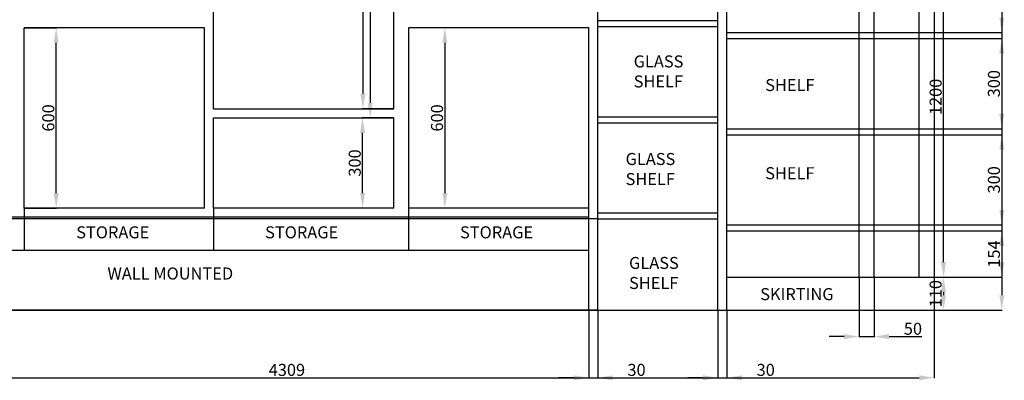
# Model space of a CAD drawing. Units: millimetres. Extents: x -2182 to 7969, y 257 to 4097.
# Tile 4 of 5: x 4692 to 7969, y 257 to 1457. Entities that reach past the tile are written whole.
import ezdxf

# ---------------------------------------------------------------- set-up
doc = ezdxf.new("R2010")
doc.units = ezdxf.units.MM
for name, color, linetype, lineweight in [('A-ANNO-DIMS', 2, 'Continuous', 18), ('A-ANNO-TEXT', 3, 'Continuous', 18), ('A-ELEV', 7, 'Continuous', 25)]:
    doc.layers.add(name, color=color, linetype=linetype, lineweight=lineweight)
doc.styles.get("Standard").update_dxf_attribs({"font": 'arial.ttf'})
doc.dimstyles.new('ISO-25', dxfattribs={"dimtxt": 40, "dimasz": 50, "dimexe": 1.25, "dimexo": 0.625, "dimtad": 1, "dimtxsty": 'Standard', "dimcen": 2.5, "dimadec": 0, "dimazin": 0, "dimtfac": 1, "dimtmove": 0, "dimatfit": 3, "dimfxl": 1, "dimarcsym": 0})

# ---------------------------------------------------------------- blocks, each defined once
blk = doc.blocks.new('*D52')
at = {"layer": 'A-ANNO-DIMS', "color": 0, "lineweight": -2, "transparency": 16777216}
for p, q in [((7686.6, 600), (7768.1, 600)), ((7766.8, 550), (7766.8, 540)), ((7686.6, 490), (7768.1, 490))]:
    blk.add_line(p, q, dxfattribs=at)
at = {"layer": 'A-ANNO-DIMS', "color": 0, "transparency": 16777216}
for points in [[(7758.5, 550), (7775.2, 550), (7766.8, 600)], [(7758.5, 540), (7775.2, 540), (7766.8, 490)]]:
    blk.add_solid(points, dxfattribs=at)
at = {"layer": 'Defpoints', "color": 0, "transparency": 16777216}
for p in [(7685.9, 600), (7685.9, 490), (7766.8, 490)]:
    blk.add_point(p, dxfattribs=at)
at = {"layer": 'A-ANNO-DIMS', "color": 0, "transparency": 16777216, "insert": (7745.8, 545), "char_height": 40, "attachment_point": 5, "rotation": 90}
blk.add_mtext('110', dxfattribs=at)
blk = doc.blocks.new('*D53')
at = {"layer": 'A-ANNO-DIMS', "color": 0, "lineweight": -2, "transparency": 16777216}
for p, q in [((7686.6, 1800), (7768.3, 1800)), ((7767.1, 650), (7767.1, 1750)), ((7536.6, 600), (7768.3, 600))]:
    blk.add_line(p, q, dxfattribs=at)
at = {"layer": 'A-ANNO-DIMS', "color": 0, "transparency": 16777216}
for points in [[(7758.7, 1750), (7775.4, 1750), (7767.1, 1800)], [(7758.7, 650), (7775.4, 650), (7767.1, 600)]]:
    blk.add_solid(points, dxfattribs=at)
at = {"layer": 'Defpoints', "color": 0, "transparency": 16777216}
for p in [(7685.9, 1800), (7767.1, 1800), (7535.9, 600)]:
    blk.add_point(p, dxfattribs=at)
at = {"layer": 'A-ANNO-DIMS', "color": 0, "transparency": 16777216, "insert": (7746, 1200), "char_height": 40, "attachment_point": 5, "rotation": 90}
blk.add_mtext('1200', dxfattribs=at)
blk = doc.blocks.new('*D54')
at = {"layer": 'A-ANNO-DIMS', "color": 0, "lineweight": -2, "transparency": 16777216}
for p, q in [((7485.9, 599.4), (7485.9, 400.8)), ((7535.9, 599.4), (7535.9, 400.8)), ((7435.9, 402.1), (7385.9, 402.1)), ((7485.9, 402.1), (7535.9, 402.1)), ((7585.9, 402.1), (7694.4, 402.1))]:
    blk.add_line(p, q, dxfattribs=at)
at = {"layer": 'A-ANNO-DIMS', "color": 0, "transparency": 16777216}
for points in [[(7435.9, 410.4), (7435.9, 393.7), (7485.9, 402.1)], [(7585.9, 410.4), (7585.9, 393.7), (7535.9, 402.1)]]:
    blk.add_solid(points, dxfattribs=at)
at = {"layer": 'Defpoints', "color": 0, "transparency": 16777216}
for p in [(7485.9, 600), (7535.9, 600), (7485.9, 402.1)]:
    blk.add_point(p, dxfattribs=at)
at = {"layer": 'A-ANNO-DIMS', "color": 0, "transparency": 16777216, "insert": (7665.2, 423.1), "char_height": 40, "attachment_point": 5}
blk.add_mtext('50', dxfattribs=at)
blk = doc.blocks.new('*D32')
at = {"layer": 'A-ANNO-DIMS', "color": 0, "lineweight": -2, "transparency": 16777216}
for p, q in [((6285.3, 1430), (6106, 1430)), ((6107.2, 1380), (6107.2, 880)), ((6285.3, 830), (6106, 830))]:
    blk.add_line(p, q, dxfattribs=at)
at = {"layer": 'A-ANNO-DIMS', "color": 0, "transparency": 16777216}
for points in [[(6098.9, 1380), (6115.6, 1380), (6107.2, 1430)], [(6098.9, 880), (6115.6, 880), (6107.2, 830)]]:
    blk.add_solid(points, dxfattribs=at)
at = {"layer": 'Defpoints', "color": 0, "transparency": 16777216}
for p in [(6285.9, 1430), (6107.2, 830), (6285.9, 830)]:
    blk.add_point(p, dxfattribs=at)
at = {"layer": 'A-ANNO-DIMS', "color": 0, "transparency": 16777216, "insert": (6086.2, 1130), "char_height": 40, "attachment_point": 5, "rotation": 90}
blk.add_mtext('600', dxfattribs=at)
blk = doc.blocks.new('*D40')
at = {"layer": 'A-ANNO-DIMS', "color": 0, "lineweight": -2, "transparency": 16777216}
for p, q in [((5936.3, 2864), (5857.3, 2864)), ((5858.6, 2814), (5858.6, 1180)), ((5936.3, 1130), (5857.3, 1130))]:
    blk.add_line(p, q, dxfattribs=at)
at = {"layer": 'A-ANNO-DIMS', "color": 0, "transparency": 16777216}
for points in [[(5850.2, 2814), (5866.9, 2814), (5858.6, 2864)], [(5850.2, 1180), (5866.9, 1180), (5858.6, 1130)]]:
    blk.add_solid(points, dxfattribs=at)
at = {"layer": 'Defpoints', "color": 0, "transparency": 16777216}
for p in [(5936.9, 2864), (5858.6, 1130), (5936.9, 1130)]:
    blk.add_point(p, dxfattribs=at)
at = {"layer": 'A-ANNO-DIMS', "color": 0, "transparency": 16777216, "insert": (5837.5, 1997), "char_height": 40, "attachment_point": 5, "rotation": 90}
blk.add_mtext('1734', dxfattribs=at)
blk = doc.blocks.new('*D33')
at = {"layer": 'A-ANNO-DIMS', "color": 0, "lineweight": -2, "transparency": 16777216}
for p, q in [((5936.3, 1997), (5833.1, 1997)), ((5834.4, 1947), (5834.4, 1210)), ((5936.3, 1160), (5833.1, 1160))]:
    blk.add_line(p, q, dxfattribs=at)
at = {"layer": 'A-ANNO-DIMS', "color": 0, "transparency": 16777216}
for points in [[(5826, 1947), (5842.7, 1947), (5834.4, 1997)], [(5826, 1210), (5842.7, 1210), (5834.4, 1160)]]:
    blk.add_solid(points, dxfattribs=at)
at = {"layer": 'Defpoints', "color": 0, "transparency": 16777216}
for p in [(5936.9, 1997), (5834.4, 1160), (5936.9, 1160)]:
    blk.add_point(p, dxfattribs=at)
at = {"layer": 'A-ANNO-DIMS', "color": 0, "transparency": 16777216, "insert": (5813.3, 1578.5), "char_height": 40, "attachment_point": 5, "rotation": 90}
blk.add_mtext('837', dxfattribs=at)
blk = doc.blocks.new('*D44')
at = {"layer": 'A-ANNO-DIMS', "color": 0, "lineweight": -2, "transparency": 16777216}
for p, q in [((5936.3, 1130), (5832.1, 1130)), ((5833.3, 880), (5833.3, 1080)), ((5936.3, 830), (5832.1, 830))]:
    blk.add_line(p, q, dxfattribs=at)
at = {"layer": 'A-ANNO-DIMS', "color": 0, "transparency": 16777216}
for points in [[(5825, 1080), (5841.7, 1080), (5833.3, 1130)], [(5825, 880), (5841.7, 880), (5833.3, 830)]]:
    blk.add_solid(points, dxfattribs=at)
at = {"layer": 'Defpoints', "color": 0, "transparency": 16777216}
for p in [(5833.3, 1130), (5936.9, 1130), (5936.9, 830)]:
    blk.add_point(p, dxfattribs=at)
at = {"layer": 'A-ANNO-DIMS', "color": 0, "transparency": 16777216, "insert": (5812.3, 980), "char_height": 40, "attachment_point": 5, "rotation": 90}
blk.add_mtext('300', dxfattribs=at)
blk = doc.blocks.new('*D47')
at = {"layer": 'A-ANNO-DIMS', "color": 0, "lineweight": -2, "transparency": 16777216}
for p, q in [((4707.6, 1430), (4814.7, 1430)), ((4813.4, 880), (4813.4, 1380)), ((4707.6, 830), (4814.7, 830))]:
    blk.add_line(p, q, dxfattribs=at)
at = {"layer": 'A-ANNO-DIMS', "color": 0, "transparency": 16777216}
for points in [[(4805.1, 1380), (4821.7, 1380), (4813.4, 1430)], [(4805.1, 880), (4821.7, 880), (4813.4, 830)]]:
    blk.add_solid(points, dxfattribs=at)
at = {"layer": 'Defpoints', "color": 0, "transparency": 16777216}
for p in [(4706.9, 1430), (4813.4, 1430), (4706.9, 830)]:
    blk.add_point(p, dxfattribs=at)
at = {"layer": 'A-ANNO-DIMS', "color": 0, "transparency": 16777216, "insert": (4792.4, 1130), "char_height": 40, "attachment_point": 5, "rotation": 90}
blk.add_mtext('600', dxfattribs=at)
blk = doc.blocks.new('*D77')
at = {"layer": 'A-ANNO-DIMS', "color": 0, "lineweight": -2, "transparency": 16777216}
for p, q in [((7735.9, 3063.4), (7735.9, 263.7)), ((3426.9, 489.4), (3426.9, 263.7)), ((3476.9, 265), (7685.9, 265))]:
    blk.add_line(p, q, dxfattribs=at)
at = {"layer": 'A-ANNO-DIMS', "color": 0, "transparency": 16777216}
for points in [[(3476.9, 273.3), (3476.9, 256.7), (3426.9, 265)], [(7685.9, 273.3), (7685.9, 256.7), (7735.9, 265)]]:
    blk.add_solid(points, dxfattribs=at)
at = {"layer": 'Defpoints', "color": 0, "transparency": 16777216}
for p in [(7735.9, 3064), (3426.9, 490), (7735.9, 265)]:
    blk.add_point(p, dxfattribs=at)
at = {"layer": 'A-ANNO-DIMS', "color": 0, "transparency": 16777216, "insert": (5581.4, 286.1), "char_height": 40, "attachment_point": 5}
blk.add_mtext('4309', dxfattribs=at)
blk = doc.blocks.new('*D79')
at = {"layer": 'A-ANNO-DIMS', "color": 0, "lineweight": -2, "transparency": 16777216}
for p, q in [((7736.6, 3164), (7962.2, 3164)), ((7960.9, 3114), (7960.9, 540)), ((3427.6, 490), (7962.2, 490))]:
    blk.add_line(p, q, dxfattribs=at)
at = {"layer": 'A-ANNO-DIMS', "color": 0, "transparency": 16777216}
for points in [[(7952.6, 3114), (7969.3, 3114), (7960.9, 3164)], [(7952.6, 540), (7969.3, 540), (7960.9, 490)]]:
    blk.add_solid(points, dxfattribs=at)
at = {"layer": 'Defpoints', "color": 0, "transparency": 16777216}
for p in [(7735.9, 3164), (3426.9, 490), (7960.9, 490)]:
    blk.add_point(p, dxfattribs=at)
at = {"layer": 'A-ANNO-DIMS', "color": 0, "transparency": 16777216, "insert": (7939.9, 1827), "char_height": 40, "attachment_point": 5, "rotation": 90}
blk.add_mtext('2674', dxfattribs=at)
blk = doc.blocks.new('*D90')
at = {"layer": 'A-ANNO-DIMS', "color": 0, "lineweight": -2, "transparency": 16777216}
for p, q in [((6585.9, 489.4), (6585.9, 263.7)), ((6615.9, 489.4), (6615.9, 263.7)), ((6535.9, 265), (6485.9, 265)), ((6585.9, 265), (6615.9, 265)), ((6665.9, 265), (6774.3, 265))]:
    blk.add_line(p, q, dxfattribs=at)
at = {"layer": 'A-ANNO-DIMS', "color": 0, "transparency": 16777216}
for points in [[(6535.9, 273.3), (6535.9, 256.7), (6585.9, 265)], [(6665.9, 273.3), (6665.9, 256.7), (6615.9, 265)]]:
    blk.add_solid(points, dxfattribs=at)
at = {"layer": 'Defpoints', "color": 0, "transparency": 16777216}
for p in [(6585.9, 490), (6615.9, 490), (6615.9, 265)]:
    blk.add_point(p, dxfattribs=at)
at = {"layer": 'A-ANNO-DIMS', "color": 0, "transparency": 16777216, "insert": (6745.1, 286.1), "char_height": 40, "attachment_point": 5}
blk.add_mtext('30', dxfattribs=at)
blk = doc.blocks.new('*D91')
at = {"layer": 'A-ANNO-DIMS', "color": 0, "lineweight": -2, "transparency": 16777216}
for p, q in [((7015.9, 489.4), (7015.9, 263.7)), ((7045.9, 489.4), (7045.9, 263.7)), ((6965.9, 265), (6915.9, 265)), ((7015.9, 265), (7045.9, 265)), ((7095.9, 265), (7204.3, 265))]:
    blk.add_line(p, q, dxfattribs=at)
at = {"layer": 'A-ANNO-DIMS', "color": 0, "transparency": 16777216}
for points in [[(6965.9, 273.3), (6965.9, 256.7), (7015.9, 265)], [(7095.9, 273.3), (7095.9, 256.7), (7045.9, 265)]]:
    blk.add_solid(points, dxfattribs=at)
at = {"layer": 'Defpoints', "color": 0, "transparency": 16777216}
for p in [(7015.9, 490), (7045.9, 490), (7045.9, 265)]:
    blk.add_point(p, dxfattribs=at)
at = {"layer": 'A-ANNO-DIMS', "color": 0, "transparency": 16777216, "insert": (7175.1, 286.1), "char_height": 40, "attachment_point": 5}
blk.add_mtext('30', dxfattribs=at)
blk = doc.blocks.new('*D95')
at = {"layer": 'A-ANNO-DIMS', "color": 0, "lineweight": -2, "transparency": 16777216}
for p, q in [((6615.3, 794), (3200.7, 794)), ((3201.9, 744), (3201.9, 540)), ((6615.3, 490), (3200.7, 490))]:
    blk.add_line(p, q, dxfattribs=at)
at = {"layer": 'A-ANNO-DIMS', "color": 0, "transparency": 16777216}
for points in [[(3193.6, 744), (3210.3, 744), (3201.9, 794)], [(3193.6, 540), (3210.3, 540), (3201.9, 490)]]:
    blk.add_solid(points, dxfattribs=at)
at = {"layer": 'Defpoints', "color": 0, "transparency": 16777216}
for p in [(6615.9, 794), (3201.9, 490), (6615.9, 490)]:
    blk.add_point(p, dxfattribs=at)
at = {"layer": 'A-ANNO-DIMS', "color": 0, "transparency": 16777216, "insert": (3180.9, 642), "char_height": 40, "attachment_point": 5, "rotation": 90}
blk.add_mtext('304', dxfattribs=at)
blk = doc.blocks.new('*D99')
at = {"layer": 'A-ANNO-DIMS', "color": 0, "lineweight": -2, "transparency": 16777216}
for p, q in [((7486.6, 1714), (7962.2, 1714)), ((7960.9, 1664), (7960.9, 1464)), ((7486.6, 1414), (7962.2, 1414))]:
    blk.add_line(p, q, dxfattribs=at)
at = {"layer": 'A-ANNO-DIMS', "color": 0, "transparency": 16777216}
for points in [[(7952.6, 1664), (7969.3, 1664), (7960.9, 1714)], [(7952.6, 1464), (7969.3, 1464), (7960.9, 1414)]]:
    blk.add_solid(points, dxfattribs=at)
at = {"layer": 'Defpoints', "color": 0, "transparency": 16777216}
for p in [(7485.9, 1714), (7485.9, 1414), (7960.9, 1414)]:
    blk.add_point(p, dxfattribs=at)
at = {"layer": 'A-ANNO-DIMS', "color": 0, "transparency": 16777216, "insert": (7939.9, 1564), "char_height": 40, "attachment_point": 5, "rotation": 90}
blk.add_mtext('300', dxfattribs=at)
blk = doc.blocks.new('*D100')
at = {"layer": 'A-ANNO-DIMS', "color": 0, "lineweight": -2, "transparency": 16777216}
for p, q in [((7486.6, 1394), (7962.2, 1394)), ((7960.9, 1344), (7960.9, 1144)), ((7486.6, 1094), (7962.2, 1094))]:
    blk.add_line(p, q, dxfattribs=at)
at = {"layer": 'A-ANNO-DIMS', "color": 0, "transparency": 16777216}
for points in [[(7952.6, 1344), (7969.3, 1344), (7960.9, 1394)], [(7952.6, 1144), (7969.3, 1144), (7960.9, 1094)]]:
    blk.add_solid(points, dxfattribs=at)
at = {"layer": 'Defpoints', "color": 0, "transparency": 16777216}
for p in [(7485.9, 1394), (7485.9, 1094), (7960.9, 1094)]:
    blk.add_point(p, dxfattribs=at)
at = {"layer": 'A-ANNO-DIMS', "color": 0, "transparency": 16777216, "insert": (7939.9, 1244), "char_height": 40, "attachment_point": 5, "rotation": 90}
blk.add_mtext('300', dxfattribs=at)
blk = doc.blocks.new('*D101')
at = {"layer": 'A-ANNO-DIMS', "color": 0, "lineweight": -2, "transparency": 16777216}
for p, q in [((7486.6, 1074), (7962.2, 1074)), ((7960.9, 1024), (7960.9, 824)), ((7486.6, 774), (7962.2, 774))]:
    blk.add_line(p, q, dxfattribs=at)
at = {"layer": 'A-ANNO-DIMS', "color": 0, "transparency": 16777216}
for points in [[(7952.6, 1024), (7969.3, 1024), (7960.9, 1074)], [(7952.6, 824), (7969.3, 824), (7960.9, 774)]]:
    blk.add_solid(points, dxfattribs=at)
at = {"layer": 'Defpoints', "color": 0, "transparency": 16777216}
for p in [(7485.9, 1074), (7485.9, 774), (7960.9, 774)]:
    blk.add_point(p, dxfattribs=at)
at = {"layer": 'A-ANNO-DIMS', "color": 0, "transparency": 16777216, "insert": (7939.9, 924), "char_height": 40, "attachment_point": 5, "rotation": 90}
blk.add_mtext('300', dxfattribs=at)
blk = doc.blocks.new('*D102')
at = {"layer": 'A-ANNO-DIMS', "color": 0, "lineweight": -2, "transparency": 16777216}
for p, q in [((7486.6, 754), (7962.2, 754)), ((7960.9, 704), (7960.9, 650)), ((7486.6, 600), (7962.2, 600))]:
    blk.add_line(p, q, dxfattribs=at)
at = {"layer": 'A-ANNO-DIMS', "color": 0, "transparency": 16777216}
for points in [[(7952.6, 704), (7969.3, 704), (7960.9, 754)], [(7952.6, 650), (7969.3, 650), (7960.9, 600)]]:
    blk.add_solid(points, dxfattribs=at)
at = {"layer": 'Defpoints', "color": 0, "transparency": 16777216}
for p in [(7485.9, 754), (7485.9, 600), (7960.9, 600)]:
    blk.add_point(p, dxfattribs=at)
at = {"layer": 'A-ANNO-DIMS', "color": 0, "transparency": 16777216, "insert": (7939.9, 677), "char_height": 40, "attachment_point": 5, "rotation": 90}
blk.add_mtext('154', dxfattribs=at)

msp = doc.modelspace()

# ---------------------------------------------------------------- linework, layer by layer
at = {"layer": 'A-ELEV'}
for p, q in [((5936.9478, 1159.9911), (5936.9478, 3163.9911)), ((7535.9478, 599.9911), (7535.9478, 3063.9911)), ((7685.9478, 599.9911), (7685.9478, 3063.9911)), ((6615.9478, 489.9911), (6615.9478, 2713.9911)), ((7015.9478, 489.9911), (7015.9478, 2713.9911)), ((7045.9478, 489.9911), (7045.9478, 2593.9911)), ((7485.9478, 599.9911), (7485.9478, 2593.9911)), ((5336.9478, 1159.9911), (5336.9478, 1996.9911)), ((6615.9478, 1453.9911), (7015.9478, 1453.9911)), ((6615.9478, 1453.9911), (7015.9478, 1453.9911)), ((4706.9478, 829.9911), (4706.9478, 1429.9911)), ((5306.9478, 1429.9911), (4706.9478, 1429.9911)), ((5306.9478, 829.9911), (5306.9478, 1429.9911)), ((5985.9478, 1429.9911), (5985.9478, 829.9911)), ((6585.9478, 1429.9911), (5985.9478, 1429.9911)), ((6585.9478, 489.9911), (6585.9478, 1429.9911)), ((6615.9478, 1433.9911), (7015.9478, 1433.9911)), ((6615.9478, 1433.9911), (7015.9478, 1433.9911)), ((7045.9478, 1413.9911), (7485.9478, 1413.9911)), ((7045.9478, 1393.9911), (7485.9478, 1393.9911)), ((5336.9478, 1159.9911), (5936.9478, 1159.9911)), ((5336.9478, 829.9911), (5336.9478, 1129.9911)), ((5336.9478, 1129.9911), (5936.9478, 1129.9911)), ((5936.9478, 829.9911), (5936.9478, 1129.9911)), ((6615.9478, 1133.9911), (7015.9478, 1133.9911)), ((6615.9478, 1133.9911), (7015.9478, 1133.9911)), ((6615.9478, 1113.9911), (7015.9478, 1113.9911)), ((6615.9478, 1113.9911), (7015.9478, 1113.9911)), ((7045.9478, 1093.9911), (7485.9478, 1093.9911)), ((7045.9478, 1073.9911), (7485.9478, 1073.9911)), ((5306.9478, 829.9911), (4706.9478, 829.9911)), ((4706.9478, 829.9911), (4706.9478, 689.9911)), ((5936.9478, 829.9911), (5336.9478, 829.9911)), ((5336.9478, 829.9911), (5336.9478, 689.9911)), ((6585.9478, 829.9911), (5985.9478, 829.9911)), ((5985.9478, 829.9911), (5985.9478, 689.9911)), ((6585.9478, 799.9911), (4076.9478, 799.9911)), ((6615.9478, 813.9911), (7015.9478, 813.9911)), ((6615.9478, 793.9911), (7015.9478, 793.9911)), ((7045.9478, 773.9911), (7485.9478, 773.9911)), ((7045.9478, 753.9911), (7485.9478, 753.9911)), ((3576.9478, 689.9911), (6585.9478, 689.9911)), ((7045.9478, 599.9911), (7485.9478, 599.9911)), ((7535.9478, 599.9911), (7685.9478, 599.9911)), ((3426.9478, 489.9911), (7685.9478, 489.9911))]:
    msp.add_line(p, q, dxfattribs=at)

# ---------------------------------------------------------------- texts
at = {"layer": 'A-ANNO-TEXT', "char_height": 40, "width": 482.986246, "attachment_point": 1}
for s, insert in [('GLASS \\PSHELF', (6735.6403, 1338.1577)), ('\\PSHELF', (7173.4129, 1326.179)), ('GLASS \\PSHELF', (6708.7107, 1013.2851)), ('\\PSHELF', (7173.4129, 1032.6915)), ('STORAGE', (4880.0838, 769.1953)), ('STORAGE', (5508.8464, 769.1953)), ('STORAGE', (6157.6701, 769.1953)), ('GLASS \\PSHELF', (6720.2515, 667.2677)), ('WALL MOUNTED', (4984.0011, 632.1675)), ('SKIRTING', (7156.8462, 563.5447))]:
    msp.add_mtext(s, dxfattribs=dict(at, insert=insert))

# ---------------------------------------------------------------- dimensions: what is measured, and where the dimension line sits
at = {"layer": 'A-ANNO-DIMS'}
for base, p1, p2, override, picture, middle in [((7960.9478, 489.9911), (7735.9478, 3163.9911), (3426.9478, 489.9911), {"dimdec": 0, "dimlfac": 1, "dimrnd": 0, "dimzin": 0, "dimdsep": 46, "dimlunit": 2}, '*D79', (7939.8999, 1826.9911)), ((5858.5641, 1129.9911), (5936.9478, 2863.9911), (5936.9478, 1129.9911), {"dimclrd": 0, "dimclre": 0, "dimclrt": 0}, '*D40', (5837.5025, 1996.9911)), ((5834.375, 1159.9911), (5936.9478, 1996.9911), (5936.9478, 1159.9911), {"dimclrd": 0, "dimclre": 0, "dimclrt": 0}, '*D33', (5813.3135, 1578.4911)), ((7767.0748, 1799.9911), (7535.9478, 599.9911), (7685.9478, 1799.9911), {"dimclrd": 0, "dimclre": 0, "dimclrt": 0}, '*D53', (7746.0269, 1199.9911)), ((7960.9478, 1413.9911), (7485.9478, 1713.9911), (7485.9478, 1413.9911), {"dimdec": 0, "dimlfac": 1, "dimrnd": 0, "dimzin": 0, "dimdsep": 46, "dimlunit": 2}, '*D99', (7939.8862, 1563.9911)), ((4813.4156, 1429.9911), (4706.9478, 829.9911), (4706.9478, 1429.9911), {"dimclrd": 0, "dimclre": 0, "dimclrt": 0}, '*D47', (4792.3677, 1129.9911)), ((6107.2476, 829.9911), (6285.9478, 1429.9911), (6285.9478, 829.9911), {"dimclrd": 0, "dimclre": 0, "dimclrt": 0}, '*D32', (6086.1996, 1129.9911)), ((7960.9478, 1093.9911), (7485.9478, 1393.9911), (7485.9478, 1093.9911), {"dimdec": 0, "dimlfac": 1, "dimrnd": 0, "dimzin": 0, "dimdsep": 46, "dimlunit": 2}, '*D100', (7939.8862, 1243.9911)), ((5833.3276, 1129.9911), (5936.9478, 829.9911), (5936.9478, 1129.9911), {"dimclrd": 0, "dimclre": 0, "dimclrt": 0}, '*D44', (5812.266, 979.9911)), ((7960.9478, 773.9911), (7485.9478, 1073.9911), (7485.9478, 773.9911), {"dimdec": 0, "dimlfac": 1, "dimrnd": 0, "dimzin": 0, "dimdsep": 46, "dimlunit": 2}, '*D101', (7939.8862, 923.9911)), ((3201.9478, 489.9911), (6615.9478, 793.9911), (6615.9478, 489.9911), {"dimdec": 0, "dimlfac": 1, "dimrnd": 0, "dimzin": 0, "dimdsep": 46, "dimlunit": 2}, '*D95', (3180.8862, 641.9911)), ((7960.9478, 599.9911), (7485.9478, 753.9911), (7485.9478, 599.9911), {"dimdec": 0, "dimlfac": 1, "dimrnd": 0, "dimzin": 0, "dimdsep": 46, "dimlunit": 2}, '*D102', (7939.8999, 676.9911))]:
    dim = msp.add_linear_dim(base=base, p1=p1, p2=p2, angle=90, dimstyle='ISO-25', override=override, dxfattribs=at)
    dim.commit()
    dim.dimension.update_dxf_attribs({"geometry": picture, "text_midpoint": middle})
for base, p1, p2, picture, middle in [((7735.9478, 264.9911), (3426.9478, 489.9911), (7735.9478, 3063.9911), '*D77', (5581.4478, 286.0526)), ((6615.9478, 264.9911), (6585.9478, 489.9911), (6615.9478, 489.9911), '*D90', (6745.1403, 286.0526)), ((7045.9478, 264.9911), (7015.9478, 489.9911), (7045.9478, 489.9911), '*D91', (7175.1403, 286.0526))]:
    dim = msp.add_linear_dim(base=base, p1=p1, p2=p2, dimstyle='ISO-25', override={"dimdec": 0, "dimlfac": 1, "dimrnd": 0, "dimzin": 0, "dimdsep": 46, "dimlunit": 2}, dxfattribs=at)
    dim.commit()
    dim.dimension.update_dxf_attribs({"geometry": picture, "text_midpoint": middle})
dim = msp.add_linear_dim(base=(7485.9478, 402.0582), p1=(7535.9478, 599.9911), p2=(7485.9478, 599.9911), dimstyle='ISO-25', override={"dimclrd": 0, "dimclre": 0, "dimclrt": 0}, dxfattribs=at)
dim.commit()
dim.dimension.update_dxf_attribs({"geometry": '*D54', "text_midpoint": (7665.154, 402.0582), "dimtype": 160})
dim = msp.add_linear_dim(base=(7766.8293, 489.9911), p1=(7685.9478, 599.9911), p2=(7685.9478, 489.9911), angle=90, dimstyle='ISO-25', override={"dimclrd": 0, "dimclre": 0, "dimclrt": 0}, dxfattribs=at)
dim.commit()
dim.dimension.update_dxf_attribs({"geometry": '*D52', "text_midpoint": (7766.8293, 544.9911), "dimtype": 160})

doc.saveas('drawing.dxf')
